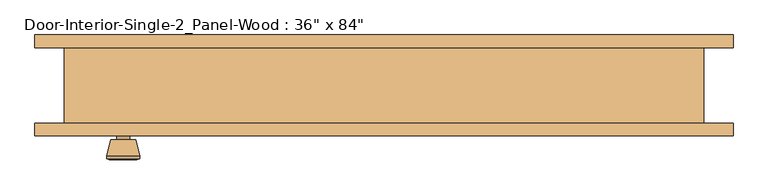
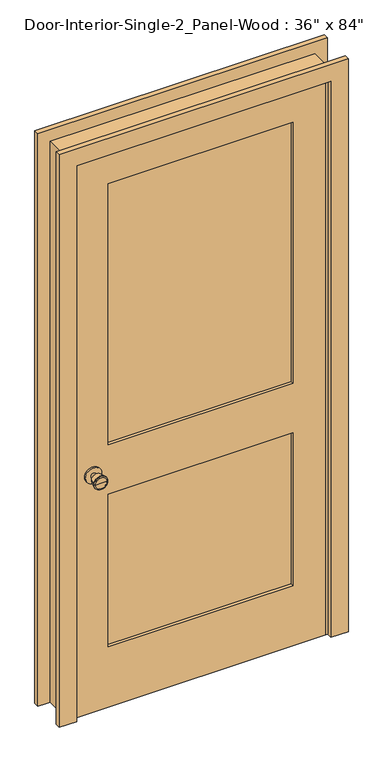
"""IFC4 building model written with IfcOpenShell, lengths in millimetres: door geometry."""

from ifc_helpers import new_model, si_unit, point, frame, frame_2d, origin, place, context, project, spatial, polyline, circle_curve, trimmed, segment, composite_curve, outline, extrude, faceted_brep, source, transform, mapped, element, save
from ifc_brep_helpers import plane_surface, cylinder_surface, revolved_surface, advanced_brep


def door_049a69ed(model_context):
    return source(origin(), model_context, "Body", "SolidModel", [
        advanced_brep(
        [(-393.7, -13.05, 914.4), (-403.7, -13.05, 914.4), (-383.7, -13.05, 914.4), (-373.2241324, 35.95, 914.4), (-414.1758676, 35.95, 914.4), (-393.7, 35.95, 914.4), (-368.7, 34.1221319, 914.4), (-418.7, 34.1221319, 914.4), (-368.7, 30.6584537, 914.4), (-418.7, 30.6584537, 914.4), (-375.063764, 5.95, 914.4), (-412.336236, 5.95, 914.4), (-383.7, 5.95, 914.4), (-403.7, 5.95, 914.4)],
        [
            (0, 1),
            (1, 2, circle_curve(frame((-393.7, -13.05, 914.4), z_axis=(0.0, -1.0, 0.0), x_axis=(-1.0, 0.0, 0.0)), 10.0)),
            (2, 0),
            (2, 1, circle_curve(frame((-393.7, -13.05, 914.4), z_axis=(0.0, -1.0, 0.0), x_axis=(-1.0, 0.0, 0.0)), 10.0)),
            (3, 4, circle_curve(frame((-393.7, 35.95, 914.4), z_axis=(0.0, 1.0, 0.0), x_axis=(-1.0, 0.0, 0.0)), 20.4758676)),
            (4, 5),
            (5, 3),
            (4, 3, circle_curve(frame((-393.7, 35.95, 914.4), z_axis=(0.0, 1.0, 0.0), x_axis=(-1.0, 0.0, 0.0)), 20.4758676)),
            (6, 7, circle_curve(frame((-393.7, 34.1221319, 914.4), z_axis=(0.0, 1.0, 0.0), x_axis=(-1.0, 0.0, 0.0)), 25.0)),
            (7, 4),
            (3, 6),
            (7, 6, circle_curve(frame((-393.7, 34.1221319, 914.4), z_axis=(0.0, 1.0, 0.0), x_axis=(-1.0, 0.0, 0.0)), 25.0)),
            (8, 9, circle_curve(frame((-393.7, 30.6584537, 914.4), z_axis=(0.0, 1.0, 0.0), x_axis=(-1.0, 0.0, 0.0)), 25.0)),
            (9, 7),
            (6, 8),
            (9, 8, circle_curve(frame((-393.7, 30.6584537, 914.4), z_axis=(0.0, 1.0, 0.0), x_axis=(-1.0, 0.0, 0.0)), 25.0)),
            (10, 11, circle_curve(frame((-393.7, 5.95, 914.4), z_axis=(0.0, 1.0, 0.0), x_axis=(-1.0, 0.0, 0.0)), 18.636236)),
            (11, 9),
            (8, 10),
            (11, 10, circle_curve(frame((-393.7, 5.95, 914.4), z_axis=(0.0, 1.0, 0.0), x_axis=(-1.0, 0.0, 0.0)), 18.636236)),
            (12, 13, circle_curve(frame((-393.7, 5.95, 914.4), z_axis=(0.0, 1.0, 0.0), x_axis=(-1.0, 0.0, 0.0)), 10.0)),
            (13, 11),
            (10, 12),
            (13, 12, circle_curve(frame((-393.7, 5.95, 914.4), z_axis=(0.0, 1.0, 0.0), x_axis=(-1.0, 0.0, 0.0)), 10.0)),
            (1, 13),
            (12, 2),
        ],
        [
            plane_surface(frame((-393.7, -13.05, 914.4), z_axis=(0.0, -1.0, 0.0), x_axis=(-1.0, 0.0, 0.0))),
            plane_surface(frame((-393.7, 35.95, 914.4), z_axis=(0.0, 1.0, 0.0), x_axis=(-1.0, 0.0, 0.0))),
            revolved_surface(polyline([(-414.1758676, 35.95, 914.4), (-418.7, 34.1221319, 914.4)]), (-393.7, -13.05, 914.4), (0.0, -1.0, 0.0)),
            cylinder_surface(frame((-393.7, -13.05, 914.4), z_axis=(0.0, -1.0, 0.0), x_axis=(-1.0, 0.0, 0.0)), 25.0),
            revolved_surface(polyline([(-418.7, 30.6584537, 914.4), (-412.336236, 5.95, 914.4)]), (-393.7, -13.05, 914.4), (0.0, -1.0, 0.0)),
            plane_surface(frame((-393.7, 5.95, 914.4), z_axis=(0.0, -1.0, 0.0), x_axis=(-1.0, 0.0, 0.0))),
            cylinder_surface(frame((-393.7, -13.05, 914.4), z_axis=(0.0, -1.0, 0.0), x_axis=(-1.0, 0.0, 0.0)), 10.0),
        ],
        [
            (0, [[1, 2, 3]]),
            (0, [[-3, 4, -1]]),
            (1, [[5, 6, 7]]),
            (1, [[8, -7, -6]]),
            (2, [[9, 10, -5, 11]]),
            (2, [[12, -11, -8, -10]]),
            (3, [[13, 14, -9, 15]]),
            (3, [[16, -15, -12, -14]]),
            (4, [[17, 18, -13, 19]]),
            (4, [[20, -19, -16, -18]]),
            (5, [[21, 22, -17, 23]]),
            (5, [[24, -23, -20, -22]]),
            (6, [[-2, 25, -21, 26]]),
            (6, [[-4, -26, -24, -25]]),
        ],
    ),
        extrude(outline(composite_curve([segment(trimmed(circle_curve(frame_2d((914.4, -393.7)), 30.0), [point((914.4, -423.7))], [point((914.4, -363.7))], False, "CARTESIAN"), True, "CONTINUOUS"), segment(trimmed(circle_curve(frame_2d((914.4, -393.7)), 30.0), [point((914.4, -363.7))], [point((914.4, -423.7))], False, "CARTESIAN"), True, "CONTINUOUS")], self_intersect=False)), frame((0.0, -19.05, 0.0), z_axis=(0.0, 1.0, 0.0), x_axis=(0.0, 0.0, 1.0)), (0.0, 0.0, 1.0), 6.0),
        advanced_brep(
        [(-393.7, -59.975, 914.4), (-383.7, -59.975, 914.4), (-403.7, -59.975, 914.4), (-373.2241324, -108.975, 914.4), (-393.7, -108.975, 914.4), (-414.1758676, -108.975, 914.4), (-368.7, -107.1471319, 914.4), (-418.7, -107.1471319, 914.4), (-368.7, -103.6834537, 914.4), (-418.7, -103.6834537, 914.4), (-375.063764, -78.975, 914.4), (-412.336236, -78.975, 914.4), (-383.7, -78.975, 914.4), (-403.7, -78.975, 914.4)],
        [
            (0, 1),
            (1, 2, circle_curve(frame((-393.7, -59.975, 914.4), z_axis=(0.0, 1.0, 0.0), x_axis=(-1.0, 0.0, 0.0)), 10.0)),
            (2, 0),
            (2, 1, circle_curve(frame((-393.7, -59.975, 914.4), z_axis=(0.0, 1.0, 0.0), x_axis=(-1.0, 0.0, 0.0)), 10.0)),
            (3, 4),
            (4, 5),
            (5, 3, circle_curve(frame((-393.7, -108.975, 914.4), z_axis=(0.0, -1.0, 0.0), x_axis=(-1.0, 0.0, 0.0)), 20.4758676)),
            (3, 5, circle_curve(frame((-393.7, -108.975, 914.4), z_axis=(0.0, -1.0, 0.0), x_axis=(-1.0, 0.0, 0.0)), 20.4758676)),
            (6, 3),
            (5, 7),
            (7, 6, circle_curve(frame((-393.7, -107.1471319, 914.4), z_axis=(0.0, -1.0, 0.0), x_axis=(-1.0, 0.0, 0.0)), 25.0)),
            (6, 7, circle_curve(frame((-393.7, -107.1471319, 914.4), z_axis=(0.0, -1.0, 0.0), x_axis=(-1.0, 0.0, 0.0)), 25.0)),
            (8, 6),
            (7, 9),
            (9, 8, circle_curve(frame((-393.7, -103.6834537, 914.4), z_axis=(0.0, -1.0, 0.0), x_axis=(-1.0, 0.0, 0.0)), 25.0)),
            (8, 9, circle_curve(frame((-393.7, -103.6834537, 914.4), z_axis=(0.0, -1.0, 0.0), x_axis=(-1.0, 0.0, 0.0)), 25.0)),
            (10, 8),
            (9, 11),
            (11, 10, circle_curve(frame((-393.7, -78.975, 914.4), z_axis=(0.0, -1.0, 0.0), x_axis=(-1.0, 0.0, 0.0)), 18.636236)),
            (10, 11, circle_curve(frame((-393.7, -78.975, 914.4), z_axis=(0.0, -1.0, 0.0), x_axis=(-1.0, 0.0, 0.0)), 18.636236)),
            (12, 10),
            (11, 13),
            (13, 12, circle_curve(frame((-393.7, -78.975, 914.4), z_axis=(0.0, -1.0, 0.0), x_axis=(-1.0, 0.0, 0.0)), 10.0)),
            (12, 13, circle_curve(frame((-393.7, -78.975, 914.4), z_axis=(0.0, -1.0, 0.0), x_axis=(-1.0, 0.0, 0.0)), 10.0)),
            (1, 12),
            (13, 2),
        ],
        [
            plane_surface(frame((-393.7, -59.975, 914.4), z_axis=(0.0, 1.0, 0.0), x_axis=(-1.0, 0.0, 0.0))),
            plane_surface(frame((-393.7, -108.975, 914.4), z_axis=(0.0, -1.0, 0.0), x_axis=(-1.0, 0.0, 0.0))),
            revolved_surface(polyline([(-414.1758676, -108.975, 914.4), (-418.7, -107.1471319, 914.4)]), (-393.7, -59.975, 914.4), (0.0, 1.0, 0.0)),
            cylinder_surface(frame((-393.7, -59.975, 914.4), z_axis=(0.0, 1.0, 0.0), x_axis=(-1.0, 0.0, 0.0)), 25.0),
            revolved_surface(polyline([(-418.7, -103.6834537, 914.4), (-412.336236, -78.975, 914.4)]), (-393.7, -59.975, 914.4), (0.0, 1.0, 0.0)),
            plane_surface(frame((-393.7, -78.975, 914.4), z_axis=(0.0, 1.0, 0.0), x_axis=(-1.0, 0.0, 0.0))),
            cylinder_surface(frame((-393.7, -59.975, 914.4), z_axis=(0.0, 1.0, 0.0), x_axis=(-1.0, 0.0, 0.0)), 10.0),
        ],
        [
            (0, [[1, 2, 3]]),
            (0, [[-3, 4, -1]]),
            (1, [[5, 6, 7]]),
            (1, [[-6, -5, 8]]),
            (2, [[9, -7, 10, 11]]),
            (2, [[-10, -8, -9, 12]]),
            (3, [[13, -11, 14, 15]]),
            (3, [[-14, -12, -13, 16]]),
            (4, [[17, -15, 18, 19]]),
            (4, [[-18, -16, -17, 20]]),
            (5, [[21, -19, 22, 23]]),
            (5, [[-22, -20, -21, 24]]),
            (6, [[25, -23, 26, -2]]),
            (6, [[-26, -24, -25, -4]]),
        ],
    ),
        extrude(outline(composite_curve([segment(trimmed(circle_curve(frame_2d((914.4, -393.7)), 30.0), [point((914.4, -423.7))], [point((914.4, -363.7))], False, "CARTESIAN"), True, "CONTINUOUS"), segment(trimmed(circle_curve(frame_2d((914.4, -393.7)), 30.0), [point((914.4, -363.7))], [point((914.4, -423.7))], False, "CARTESIAN"), True, "CONTINUOUS")], self_intersect=False)), frame((0.0, -59.975, 0.0), z_axis=(0.0, 1.0, 0.0), x_axis=(0.0, 0.0, 1.0)), (0.0, 0.0, 1.0), 6.0),
        faceted_brep([(482.6, -53.975, 0.0), (457.2, -53.975, 0.0), (457.2, -19.05, 0.0), (444.5, -19.05, 0.0), (444.5, 15.875, 0.0), (457.2, 15.875, 0.0), (457.2, 60.325, 0.0), (482.6, 60.325, 0.0), (482.6, 60.325, 2159.0), (482.6, -53.975, 2159.0), (457.2, 60.325, 2133.6), (-457.2, 60.325, 2133.6), (-457.2, 60.325, 0.0), (-482.6, 60.325, 0.0), (-482.6, 60.325, 2159.0), (457.2, 15.875, 2133.6), (444.5, 15.875, 2120.9), (-444.5, 15.875, 2120.9), (-444.5, 15.875, 0.0), (-457.2, 15.875, 0.0), (-457.2, 15.875, 2133.6), (444.5, -19.05, 2120.9), (457.2, -19.05, 2133.6), (-457.2, -19.05, 2133.6), (-457.2, -19.05, 0.0), (-444.5, -19.05, 0.0), (-444.5, -19.05, 2120.9), (457.2, -53.975, 2133.6), (-482.6, -53.975, 2159.0), (-482.6, -53.975, 0.0), (-457.2, -53.975, 0.0), (-457.2, -53.975, 2133.6)], [[[0, 1, 2, 3, 4, 5, 6, 7]], [[7, 8, 9, 0]], [[6, 10, 11, 12, 13, 14, 8, 7]], [[5, 15, 10, 6]], [[4, 16, 17, 18, 19, 20, 15, 5]], [[3, 21, 16, 4]], [[2, 22, 23, 24, 25, 26, 21, 3]], [[1, 27, 22, 2]], [[0, 9, 28, 29, 30, 31, 27, 1]], [[8, 14, 28, 9]], [[15, 20, 11, 10]], [[21, 26, 17, 16]], [[27, 31, 23, 22]], [[29, 13, 12, 19, 18, 25, 24, 30]], [[14, 13, 29, 28]], [[20, 19, 12, 11]], [[26, 25, 18, 17]], [[31, 30, 24, 23]]]),
        extrude(outline(polyline([(2133.6, -457.2), (0.0, -457.2), (0.0, 457.2), (2133.6, 457.2), (2133.6, -457.2)]), holes=[polyline([(2014.5375, -336.55), (2014.5375, 336.55), (1009.65, 336.55), (1009.65, -336.55), (2014.5375, -336.55)]), polyline([(819.15, -336.55), (819.15, 336.55), (231.775, 336.55), (231.775, -336.55), (819.15, -336.55)])]), frame((0.0, -53.975, 0.0), z_axis=(0.0, 1.0, 0.0), x_axis=(0.0, 0.0, 1.0)), (0.0, 0.0, 1.0), 34.925),
        extrude(outline(polyline([(336.55, -30.6916667), (336.55, -42.3333333), (-336.55, -42.3333333), (-336.55, -30.6916667), (336.55, -30.6916667)])), frame((0.0, 0.0, 1009.65), z_axis=(0.0, 0.0, 1.0), x_axis=(1.0, 0.0, 0.0)), (0.0, 0.0, 1.0), 1004.8875),
        extrude(outline(polyline([(336.55, -30.6916667), (336.55, -42.3333333), (-336.55, -42.3333333), (-336.55, -30.6916667), (336.55, -30.6916667)])), frame((0.0, 0.0, 231.775), z_axis=(0.0, 0.0, 1.0), x_axis=(1.0, 0.0, 0.0)), (0.0, 0.0, 1.0), 587.375),
        extrude(outline(polyline([(0.0, 527.05), (2203.45, 527.05), (2203.45, -527.05), (0.0, -527.05), (0.0, -463.55), (2139.95, -463.55), (2139.95, 463.55), (0.0, 463.55), (0.0, 527.05)])), frame((0.0, -73.025, 0.0), z_axis=(0.0, 1.0, 0.0), x_axis=(0.0, 0.0, 1.0)), (0.0, 0.0, 1.0), 19.05),
        extrude(outline(polyline([(0.0, 527.05), (2203.45, 527.05), (2203.45, -527.05), (0.0, -527.05), (0.0, -463.55), (2139.95, -463.55), (2139.95, 463.55), (0.0, 463.55), (0.0, 527.05)])), frame((0.0, 60.325, 0.0), z_axis=(0.0, 1.0, 0.0), x_axis=(0.0, 0.0, 1.0)), (0.0, 0.0, 1.0), 19.05),
    ])


if __name__ == "__main__":
    model = new_model("IFC4")
    model_context = context("Model", 3, world=origin())
    ifc_project = project(units=[si_unit("LENGTHUNIT", "METRE", prefix="MILLI")], contexts=[model_context])
    site = spatial("IfcSite", under=ifc_project)
    building = spatial("IfcBuilding", under=site)
    placement = place(None, origin())
    door_shape = door_049a69ed(model_context)
    element("IfcDoor", 1, ObjectType="Door-Interior-Single-2_Panel-Wood : 36\" x 84\"", at=placement, inside=building, context=model_context, shape_type="MappedRepresentation", body=[
        mapped(door_shape, transform((0.0, 0.0, 0.0), x_axis=(1.0, 0.0, 0.0), y_axis=(0.0, 1.0, 0.0), z_axis=(0.0, 0.0, 1.0))),
    ])
    save(model, "model.ifc")

# Revit data of these elements
# Type "Door-Interior-Single-2_Panel-Wood : 36\" x 84\""
#   Type Mark = "9"
#   Assembly Code = "C1020300"
#   Analytic Construction = "Wooden"
#   Top Rail = 0' - 4 11/16"
#   Thickness = 0' - 1 3/8"
#   Thermal Resistance (R) = 2.5876 (h·ft²·°F)/BTU
#   Swing Angle [instance default] = 90.00°
#   Stiles = 0' - 4 3/4"
#   Rough Width = 3' - 2"
#   Rough Height = 7' - 1"
#   Lock Rail = 0' - 7 1/2"
#   Height = 7' - 0"
#   Width = 3' - 0"
#   Heat Transfer Coefficient (U) = 0.3865 BTU/(h·ft²·°F)
#   Bottom Rail = 0' - 9 1/8"
#   Trim Material = Cherry
#   Panel Material = Cherry
#   Frame Material = Cherry
#   Door Handle Material = Aluminum
#   Visual Light Transmittance = 0
#   Solar Heat Gain Coefficient = 0
#   Wall Closure = (empty or 0)
#   Function = (empty or 0)
# Element 1 (IfcDoor, "Door-Interior-Single-2_Panel-Wood : 36\" x 84\"")
#   Materials on its faces: "Cherry", "Aluminum"
# Materials
#   "Cherry": class "Wood", colour RGB 226 177 128, transparency 0, Description = "Prunus Serotina", Cost = 0
#   "Aluminum": class "Metal", colour RGB 247 247 247, transparency 0, Description = "Aluminum 6061", Cost = 0
